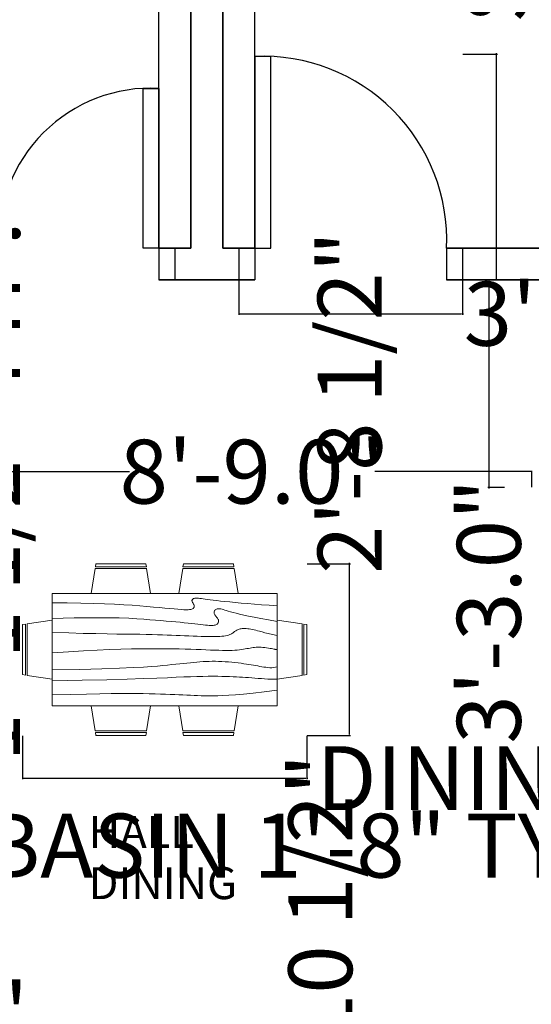
# Model space of a CAD drawing. Units: inches. Extents: x -52 to 472, y -40 to 644.
# Tile 4 of 6: x 154 to 250, y 164 to 349. Entities that reach past the tile are written whole.
import ezdxf

# ---------------------------------------------------------------- set-up
doc = ezdxf.new("R2010")
doc.units = ezdxf.units.IN
doc.header["$MEASUREMENT"] = 0
for name, color, linetype, lineweight in [('A-ANNO-DIMS', 7, 'Continuous', 13), ('A-ANNO-TEXT', 7, 'Continuous', 18), ('DOORS', 2, 'Continuous', 25), ('FURNITURE', 6, 'Continuous', 13), ('INNER WALL', 1, 'Continuous', 35)]:
    doc.layers.add(name, color=color, linetype=linetype, lineweight=lineweight)
doc.styles.get("Standard").update_dxf_attribs({"font": 'arial.ttf'})
doc.dimstyles.get("Standard").update_dxf_attribs({"dimtxt": 12, "dimasz": 0.18, "dimexe": 0.18, "dimexo": 0.0625, "dimgap": 0.09, "dimtad": 0, "dimdec": 1, "dimzin": 0, "dimdsep": 46, "dimlunit": 3, "dimtxsty": 'Standard', "dimcen": 0.09, "dimadec": 0, "dimazin": 0, "dimtfac": 1, "dimtdec": 1, "dimtofl": 0, "dimtmove": 0, "dimatfit": 3, "dimfxl": 1, "dimtolj": 1, "dimtzin": 0, "dimarcsym": 0})

# ---------------------------------------------------------------- blocks, each defined once
blk = doc.blocks.new('Dining Set - 36 x 72 in.')
for p, q in [((-22.2343, 26.00059), (-23.4847, 17.99762)), ((-22.2304, 26), (-5.7608, 26)), ((-22, 27.5), (-22.1562, 26.50042)), ((-5.8416, 26.5), (-22.1534, 26.5)), ((-22, 27.5), (-6, 27.5)), ((-5.8437, 26.49966), (-6, 27.5)), ((-4.5152, 17.99762), (-5.7655, 25.99926)), ((5.7657, 26.00059), (4.5153, 17.99762)), ((5.7696, 26), (22.2392, 26)), ((6, 27.5), (5.8438, 26.50042)), ((22.1584, 26.5), (5.8466, 26.5)), ((6, 27.5), (22, 27.5)), ((22.1563, 26.49966), (22, 27.5)), ((23.4848, 17.99762), (22.2345, 25.99926)), ((36, 18), (-36, 18)), ((-36, 18), (-36, -18)), ((36, -18), (36, 18)), ((-44.0006, 8.23428), (-35.9976, 9.48474)), ((44.0006, 8.23428), (35.9976, 9.48474)), ((-45.5, 8), (-44.5004, 8.15617)), ((-45.5, 8), (-45.5, -8)), ((-44.5, -8.15843), (-44.5, 8.15338)), ((-44, 8.23041), (-44, -8.23915)), ((44, 8.23041), (44, -8.23915)), ((44.5, -8.15843), (44.5, 8.15338)), ((45.5, 8), (44.5005, 8.15617)), ((45.5, 8), (45.5, -8)), ((-44.4997, -8.15631), (-45.5, -8)), ((-35.9976, -9.48476), (-43.9993, -8.2345)), ((35.9976, -9.48476), (43.9993, -8.2345)), ((44.4997, -8.15631), (45.5, -8)), ((-36, -18), (36, -18)), ((-22.2343, -26.0006), (-23.4847, -17.99762)), ((-4.5152, -17.99762), (-5.7655, -25.99928)), ((5.7657, -26.0006), (4.5153, -17.99762)), ((23.4848, -17.99762), (22.2345, -25.99928)), ((-22.2304, -26), (-5.7608, -26)), ((-22, -27.5), (-22.1562, -26.50044)), ((-5.8416, -26.5), (-22.1534, -26.5)), ((-22, -27.5), (-6, -27.5)), ((-5.8437, -26.49967), (-6, -27.5)), ((5.7696, -26), (22.2392, -26)), ((6, -27.5), (5.8438, -26.50044)), ((22.1584, -26.5), (5.8466, -26.5)), ((6, -27.5), (22, -27.5)), ((22.1563, -26.49967), (22, -27.5))]:
    blk.add_line(p, q)
for points in [[(-36, 15), (-31.1772, 14.97754), (-26.8079, 14.91406), (-22.8538, 14.81543), (-19.276, 14.6875), (-16.0362, 14.53613), (-13.0957, 14.36718), (-10.4159, 14.18652), (-7.9583, 14), (-5.6904, 13.81315), (-3.6035, 13.63021), (-1.6954, 13.45508), (0.0365, 13.29166), (1.5945, 13.14388), (2.9811, 13.01562), (4.1988, 12.9108), (5.25, 12.83333), (6.1393, 12.78613), (6.8802, 12.76823), (7.4883, 12.77767), (7.9792, 12.8125), (8.3685, 12.87077), (8.6719, 12.95052), (8.9049, 13.0498), (9.0833, 13.16666), (9.2205, 13.29899), (9.3216, 13.44401), (9.3895, 13.59879), (9.4271, 13.76041), (9.4373, 13.92594), (9.4232, 14.09245), (9.3875, 14.257), (9.3333, 14.41666), (9.2638, 14.56917), (9.1836, 14.71484), (9.0975, 14.85465), (9.0104, 14.98958), (8.9272, 15.1206), (8.8529, 15.2487), (8.7922, 15.37483), (8.75, 15.5), (8.7305, 15.62467), (8.7344, 15.74739), (8.7617, 15.86621), (8.8125, 15.97916), (8.8867, 16.08431), (8.9844, 16.17968), (9.1055, 16.26334), (9.25, 16.33333), (9.4189, 16.38802), (9.6172, 16.42708), (9.8506, 16.45052), (10.125, 16.45833), (10.4463, 16.45052), (10.8203, 16.42708), (11.2529, 16.38802), (11.75, 16.33333), (12.3184, 16.26318), (12.9694, 16.17838), (13.7151, 16.07991), (14.5677, 15.96875), (15.5395, 15.84586), (16.6426, 15.71224), (17.8893, 15.56884), (19.2917, 15.41666), (20.859, 15.25667), (22.5879, 15.08984), (24.4721, 14.91715), (26.5052, 14.73958), (28.6809, 14.5581), (30.9929, 14.3737), (33.4347, 14.18733), (36, 14)], [(-36, 10), (-28.9766, 10.14274), (-23.1725, 10.20442), (-18.4241, 10.19775), (-14.5677, 10.13541), (-11.4399, 10.03011), (-8.877, 9.89453), (-6.7154, 9.74137), (-4.7917, 9.58333), (-2.9698, 9.43082), (-1.2246, 9.28515), (0.4415, 9.14534), (2.026, 9.01041), (3.5266, 8.87939), (4.9408, 8.7513), (6.266, 8.62516), (7.5, 8.5), (8.6411, 8.37549), (9.6914, 8.2539), (10.6538, 8.13818), (11.5312, 8.03125), (12.3267, 7.93603), (13.043, 7.85547), (13.6831, 7.79248), (14.25, 7.75), (14.7471, 7.7303), (15.1797, 7.73307), (15.5537, 7.75732), (15.875, 7.80208), (16.1494, 7.86637), (16.3828, 7.94922), (16.5811, 8.04964), (16.75, 8.16666), (16.8944, 8.29915), (17.0143, 8.44531), (17.1089, 8.60319), (17.1771, 8.77083), (17.218, 8.94629), (17.2305, 9.1276), (17.2137, 9.31282), (17.1667, 9.5), (17.0895, 9.6875), (16.987, 9.875), (16.8649, 10.0625), (16.7292, 10.25), (16.5856, 10.4375), (16.4401, 10.625), (16.2985, 10.8125), (16.1667, 11), (16.05, 11.18733), (15.9518, 11.3737), (15.8752, 11.5581), (15.8229, 11.73958), (15.798, 11.91715), (15.8034, 12.08984), (15.842, 12.25667), (15.9167, 12.41666), (16.0295, 12.56836), (16.1784, 12.70833), (16.3605, 12.83268), (16.5729, 12.9375), (16.8127, 13.01888), (17.0768, 13.07291), (17.3625, 13.0957), (17.6667, 13.08333), (17.9894, 13.03312), (18.3418, 12.94726), (18.7382, 12.82918), (19.1927, 12.68229), (19.7195, 12.51001), (20.3327, 12.31575), (21.0465, 12.10294), (21.875, 11.875), (22.8357, 11.63354), (23.959, 11.37304), (25.2786, 11.08618), (26.8282, 10.76562), (28.6414, 10.40405), (30.752, 9.99414), (33.1936, 9.52856), (36, 9)], [(-36, 5.5), (-30.7157, 5.3348), (-26.069, 5.20963), (-21.9946, 5.11767), (-18.4271, 5.05208), (-15.3009, 5.00602), (-12.5508, 4.97265), (-10.1112, 4.94515), (-7.9167, 4.91666), (-5.909, 4.88167), (-4.0586, 4.83984), (-2.3429, 4.79215), (-0.7396, 4.73958), (0.7739, 4.6831), (2.22, 4.6237), (3.6213, 4.56233), (5, 4.5), (6.373, 4.43782), (7.7344, 4.3776), (9.0723, 4.32129), (10.375, 4.27083), (11.6309, 4.22819), (12.8281, 4.19531), (13.9551, 4.17415), (15, 4.16666), (15.954, 4.17448), (16.819, 4.19791), (17.6001, 4.23698), (18.3021, 4.29166), (18.9299, 4.36198), (19.4883, 4.44791), (19.9823, 4.54948), (20.4167, 4.66666), (20.7969, 4.79899), (21.1302, 4.94401), (21.4245, 5.09879), (21.6875, 5.26041), (21.9271, 5.42594), (22.1511, 5.59245), (22.3672, 5.757), (22.5834, 5.91666), (22.8065, 6.06868), (23.0404, 6.21093), (23.2879, 6.34147), (23.5521, 6.45833), (23.8358, 6.55957), (24.142, 6.64323), (24.4735, 6.70735), (24.8334, 6.75), (25.2235, 6.76969), (25.642, 6.76692), (26.0858, 6.74267), (26.5521, 6.69791), (27.0379, 6.63362), (27.5404, 6.55078), (28.0565, 6.45036), (28.5834, 6.33333), (29.1242, 6.19987), (29.7071, 6.04687), (30.3661, 5.87044), (31.1354, 5.66666), (32.0493, 5.43164), (33.142, 5.16146), (34.4475, 4.85221), (36, 4.5)], [(-36, -1), (-30.7915, -0.6591), (-26.0195, -0.38216), (-21.6519, -0.16284), (-17.6563, 0.00521), (-14.0005, 0.12833), (-10.6523, 0.21289), (-7.5796, 0.26522), (-4.75, 0.29166), (-2.134, 0.29793), (0.2878, 0.28711), (2.5317, 0.26163), (4.6146, 0.22396), (6.5529, 0.17651), (8.3633, 0.12174), (10.0623, 0.06209), (11.6667, 0), (13.1899, -0.06201), (14.6341, -0.1211), (15.9982, -0.17432), (17.2813, -0.21875), (18.4823, -0.25147), (19.6003, -0.26953), (20.6343, -0.27002), (21.5834, -0.25), (22.4481, -0.20768), (23.2357, -0.14584), (23.9549, -0.06836), (24.6146, 0.02083), (25.2235, 0.11784), (25.7904, 0.21875), (26.3241, 0.31966), (26.8334, 0.41666), (27.3265, 0.50618), (27.8099, 0.58593), (28.2894, 0.65397), (28.7709, 0.70833), (29.2601, 0.74707), (29.763, 0.76823), (30.2855, 0.76985), (30.8334, 0.75), (31.4088, 0.70784), (31.9994, 0.64713), (32.589, 0.57275), (33.1615, 0.48958), (33.7008, 0.4025), (34.1908, 0.3164), (34.6153, 0.23616), (34.9584, 0.16666), (35.2099, 0.11165), (35.3848, 0.07031), (35.504, 0.04069), (35.5886, 0.02083), (35.6594, 0.00879), (35.7377, 0.0026), (35.8442, 0.00032), (36, 0)], [(-36, -6.5), (-27.1843, -6.31267), (-20.084, -6.1263), (-14.469, -5.9419), (-10.1094, -5.76042), (-6.7752, -5.58285), (-4.2363, -5.41016), (-2.2629, -5.24333), (-0.625, -5.08334), (0.8708, -4.93099), (2.2715, -4.78646), (3.5872, -4.64974), (4.8281, -4.52084), (6.0046, -4.39974), (7.127, -4.28646), (8.2053, -4.18099), (9.25, -4.08334), (10.2705, -3.99382), (11.2734, -3.91407), (12.2647, -3.84603), (13.25, -3.79167), (14.2354, -3.75293), (15.2266, -3.73177), (16.2295, -3.73015), (17.25, -3.75), (18.2912, -3.79248), (19.3451, -3.85547), (20.4009, -3.93604), (21.4479, -4.03125), (22.4754, -4.13819), (23.4727, -4.25391), (24.4289, -4.37549), (25.3334, -4.5), (26.1785, -4.62492), (26.9694, -4.74935), (27.7145, -4.87281), (28.4219, -4.99479), (29.1, -5.11483), (29.7572, -5.23242), (30.4016, -5.34709), (31.0417, -5.45834), (31.6837, -5.56437), (32.3262, -5.65821), (32.9658, -5.73153), (33.599, -5.77604), (34.2224, -5.78345), (34.8327, -5.74545), (35.4264, -5.65373), (36, -5.5)], [(-36, -10), (-26.4022, -9.81299), (-18.4675, -9.62891), (-11.9839, -9.45069), (-6.7396, -9.28125), (-2.5226, -9.12354), (0.8789, -8.98047), (3.6769, -8.85498), (6.0833, -8.75), (8.2767, -8.66765), (10.3021, -8.60677), (12.1712, -8.56543), (13.8958, -8.54167), (15.4876, -8.53353), (16.9583, -8.53907), (18.3197, -8.55632), (19.5834, -8.58334), (20.7616, -8.61841), (21.8685, -8.66081), (22.9188, -8.71004), (23.9271, -8.76563), (24.9081, -8.82707), (25.8763, -8.89388), (26.8465, -8.96558), (27.8334, -9.04167), (28.8474, -9.12118), (29.8828, -9.20117), (30.93, -9.27824), (31.9792, -9.34896), (33.0205, -9.40991), (34.0443, -9.45768), (35.0407, -9.48885), (36, -9.5)], [(-36, -14.5), (-30.0881, -14.33513), (-25.0332, -14.21224), (-20.7312, -14.12647), (-17.0781, -14.07292), (-13.97, -14.04671), (-11.3027, -14.04297), (-8.9724, -14.05681), (-6.875, -14.08334), (-4.9224, -14.11833), (-3.0905, -14.16016), (-1.3709, -14.20785), (0.2448, -14.26042), (1.7647, -14.3169), (3.1973, -14.3763), (4.5507, -14.43767), (5.8333, -14.5), (7.0554, -14.5621), (8.235, -14.62175), (9.3922, -14.67652), (10.5469, -14.72396), (11.7192, -14.76164), (12.929, -14.78711), (14.1965, -14.79794), (15.5417, -14.79167), (16.9933, -14.76424), (18.6152, -14.70508), (20.4804, -14.60197), (22.6615, -14.44271), (25.2312, -14.21509), (28.2624, -13.9069), (31.8277, -13.50594), (36, -13)]]:
    blk.add_lwpolyline(points)
blk = doc.blocks.new('*D15')
at = {"layer": 'A-ANNO-DIMS', "color": 0, "lineweight": -2, "transparency": 16777216}
for p, q in [((145.13, 258.39), (145.13, 264.49)), ((145.31, 264.31), (174.59, 264.31)), ((249.95, 264.31), (220.67, 264.31)), ((250.13, 261.39), (250.13, 264.49))]:
    blk.add_line(p, q, dxfattribs=at)
at = {"layer": 'A-ANNO-DIMS', "color": 0, "transparency": 16777216}
for points in [[(145.31, 264.34), (145.31, 264.28), (145.13, 264.31)], [(249.95, 264.34), (249.95, 264.28), (250.13, 264.31)]]:
    blk.add_solid(points, dxfattribs=at)
at = {"layer": 'Defpoints', "color": 0, "transparency": 16777216}
for p in [(250.13, 264.31), (250.13, 261.33), (145.13, 258.33)]:
    blk.add_point(p, dxfattribs=at)
at = {"layer": 'A-ANNO-DIMS', "color": 0, "transparency": 16777216, "insert": (197.63, 264.31), "char_height": 12, "attachment_point": 5}
blk.add_mtext('\\A1;8\'-9.0"', dxfattribs=at)
blk = doc.blocks.new('*D17')
at = {"layer": 'A-ANNO-DIMS', "color": 0, "lineweight": -2, "transparency": 16777216}
for p, q in [((32.13, 162.39), (32.13, 162.51)), ((32.31, 162.33), (89.84, 162.33)), ((210.95, 162.33), (153.42, 162.33)), ((211.13, 162.39), (211.13, 162.51))]:
    blk.add_line(p, q, dxfattribs=at)
at = {"layer": 'A-ANNO-DIMS', "color": 0, "transparency": 16777216}
for points in [[(32.31, 162.36), (32.31, 162.3), (32.13, 162.33)], [(210.95, 162.36), (210.95, 162.3), (211.13, 162.33)]]:
    blk.add_solid(points, dxfattribs=at)
at = {"layer": 'Defpoints', "color": 0, "transparency": 16777216}
for p in [(32.13, 162.33), (32.13, 162.33), (211.13, 162.33)]:
    blk.add_point(p, dxfattribs=at)
at = {"layer": 'A-ANNO-DIMS', "color": 0, "transparency": 16777216, "insert": (121.63, 162.33), "char_height": 12, "attachment_point": 5}
blk.add_mtext('\\A1;14\'-11.0"', dxfattribs=at)
blk = doc.blocks.new('*D18')
at = {"layer": 'A-ANNO-DIMS', "color": 0, "lineweight": -2, "transparency": 16777216}
for p, q in [((245, 300.33), (241.89, 300.33)), ((242.07, 300.15), (242.07, 261.49)), ((245, 261.31), (241.89, 261.31)), ((242.07, 261.31), (242.07, 261.13))]:
    blk.add_line(p, q, dxfattribs=at)
at = {"layer": 'A-ANNO-DIMS', "color": 0, "transparency": 16777216}
for points in [[(242.04, 300.15), (242.1, 300.15), (242.07, 300.33)], [(242.04, 261.49), (242.1, 261.49), (242.07, 261.31)]]:
    blk.add_solid(points, dxfattribs=at)
at = {"layer": 'Defpoints', "color": 0, "transparency": 16777216}
for p in [(245.07, 300.33), (242.07, 261.31), (245.07, 261.31)]:
    blk.add_point(p, dxfattribs=at)
at = {"layer": 'A-ANNO-DIMS', "color": 0, "transparency": 16777216, "insert": (242.07, 238.1), "char_height": 12, "attachment_point": 5, "rotation": 90}
blk.add_mtext('\\A1;3\'-3.0"', dxfattribs=at)
blk = doc.blocks.new('DOOR-36IN-SINGLE')
for p, q in [((0, 6), (0, 0)), ((3, 6), (3, 0)), ((39, 6), (39, 0)), ((42, 6), (42, 0))]:
    blk.add_line(p, q)
blk.add_lwpolyline([(3, 6), (6, 6), (6, 42), (3, 42)], close=True)
blk.add_arc((4.5, 7.5), 34.53, 357.5104, 92.4896)
blk = doc.blocks.new('*D32')
at = {"layer": 'A-ANNO-DIMS', "color": 0, "lineweight": -2, "transparency": 16777216}
for p, q in [((125.1, 196.98), (125.1, 193.87)), ((145.03, 196.98), (145.03, 193.87)), ((125.28, 194.05), (144.85, 194.05)), ((145.03, 194.05), (145.21, 194.05))]:
    blk.add_line(p, q, dxfattribs=at)
at = {"layer": 'A-ANNO-DIMS', "color": 0, "transparency": 16777216}
for points in [[(125.28, 194.08), (125.28, 194.02), (125.1, 194.05)], [(144.85, 194.08), (144.85, 194.02), (145.03, 194.05)]]:
    blk.add_solid(points, dxfattribs=at)
at = {"layer": 'Defpoints', "color": 0, "transparency": 16777216}
for p in [(125.1, 197.04), (145.03, 197.04), (145.03, 194.05)]:
    blk.add_point(p, dxfattribs=at)
at = {"layer": 'A-ANNO-DIMS', "color": 0, "transparency": 16777216, "insert": (209.09, 194.05), "char_height": 12, "attachment_point": 5}
blk.add_mtext('\\A1;BASIN 1\'-8" TYP.', dxfattribs=at)
blk = doc.blocks.new('*D33')
at = {"layer": 'A-ANNO-DIMS', "color": 0, "lineweight": -2, "transparency": 16777216}
for p, q in [((145.09, 210.33), (148.2, 210.33)), ((148.02, 210.33), (148.02, 210.51)), ((148.02, 197.22), (148.02, 210.15)), ((145.09, 197.04), (148.2, 197.04))]:
    blk.add_line(p, q, dxfattribs=at)
at = {"layer": 'A-ANNO-DIMS', "color": 0, "transparency": 16777216}
for points in [[(147.99, 210.15), (148.05, 210.15), (148.02, 210.33)], [(147.99, 197.22), (148.05, 197.22), (148.02, 197.04)]]:
    blk.add_solid(points, dxfattribs=at)
at = {"layer": 'Defpoints', "color": 0, "transparency": 16777216}
for p in [(145.03, 210.33), (148.02, 210.33), (145.03, 197.04)]:
    blk.add_point(p, dxfattribs=at)
at = {"layer": 'A-ANNO-DIMS', "color": 0, "transparency": 16777216, "insert": (148.02, 260.59), "char_height": 12, "attachment_point": 5, "rotation": 90}
blk.add_mtext('\\A1;1\'-1 1/2" TYP.', dxfattribs=at)
blk = doc.blocks.new('*D44')
at = {"layer": 'A-ANNO-DIMS', "color": 0, "lineweight": -2, "transparency": 16777216}
for p, q in [((210.42, 92.41), (210.42, 92.59)), ((217.37, 92.41), (210.24, 92.41)), ((210.42, 45.85), (210.42, 92.23)), ((217.37, 45.67), (210.24, 45.67))]:
    blk.add_line(p, q, dxfattribs=at)
at = {"layer": 'A-ANNO-DIMS', "color": 0, "transparency": 16777216}
for points in [[(210.39, 92.23), (210.45, 92.23), (210.42, 92.41)], [(210.39, 45.85), (210.45, 45.85), (210.42, 45.67)]]:
    blk.add_solid(points, dxfattribs=at)
at = {"layer": 'Defpoints', "color": 0, "transparency": 16777216}
for p in [(210.42, 92.41), (217.43, 92.41), (217.43, 45.67)]:
    blk.add_point(p, dxfattribs=at)
at = {"layer": 'A-ANNO-DIMS', "color": 0, "transparency": 16777216, "insert": (210.42, 152.12), "char_height": 12, "attachment_point": 5, "rotation": 90}
blk.add_mtext('\\A1;DESK 3\'-10 1/2"', dxfattribs=at)
blk = doc.blocks.new('*D50')
at = {"layer": 'A-ANNO-DIMS', "color": 0, "lineweight": -2, "transparency": 16777216}
for p, q in [((237.19, 342.75), (243.68, 342.75)), ((243.5, 342.75), (243.5, 342.93)), ((243.5, 300.51), (243.5, 342.57)), ((237.19, 300.33), (243.68, 300.33))]:
    blk.add_line(p, q, dxfattribs=at)
at = {"layer": 'A-ANNO-DIMS', "color": 0, "transparency": 16777216}
for points in [[(243.47, 342.57), (243.53, 342.57), (243.5, 342.75)], [(243.47, 300.51), (243.53, 300.51), (243.5, 300.33)]]:
    blk.add_solid(points, dxfattribs=at)
at = {"layer": 'Defpoints', "color": 0, "transparency": 16777216}
for p in [(237.13, 342.75), (243.5, 342.75), (237.13, 300.33)]:
    blk.add_point(p, dxfattribs=at)
at = {"layer": 'A-ANNO-DIMS', "color": 0, "transparency": 16777216, "insert": (243.5, 454.09), "char_height": 12, "attachment_point": 5, "rotation": 90}
blk.add_mtext('\\A1;SINGLE DOOR 3\'-6 1/2" TYP.', dxfattribs=at)
blk = doc.blocks.new('*D51')
at = {"layer": 'A-ANNO-DIMS', "color": 0, "lineweight": -2, "transparency": 16777216}
for p, q in [((195.13, 300.27), (195.13, 293.79)), ((237.13, 300.27), (237.13, 293.79)), ((195.31, 293.97), (236.95, 293.97)), ((237.13, 293.97), (237.31, 293.97))]:
    blk.add_line(p, q, dxfattribs=at)
at = {"layer": 'A-ANNO-DIMS', "color": 0, "transparency": 16777216}
for points in [[(195.31, 294), (195.31, 293.94), (195.13, 293.97)], [(236.95, 294), (236.95, 293.94), (237.13, 293.97)]]:
    blk.add_solid(points, dxfattribs=at)
at = {"layer": 'Defpoints', "color": 0, "transparency": 16777216}
for p in [(195.13, 300.33), (237.13, 300.33), (237.13, 293.97)]:
    blk.add_point(p, dxfattribs=at)
at = {"layer": 'A-ANNO-DIMS', "color": 0, "transparency": 16777216, "insert": (273.97, 293.97), "char_height": 12, "attachment_point": 5}
blk.add_mtext('\\A1;3\'-6" TYP.', dxfattribs=at)
blk = doc.blocks.new('*D52')
at = {"layer": 'A-ANNO-DIMS', "color": 0, "lineweight": -2, "transparency": 16777216}
for p, q in [((123.77, 136.75), (123.77, 136.93)), ((130.07, 136.75), (123.59, 136.75)), ((123.77, 94.51), (123.77, 136.57)), ((130.07, 94.33), (123.59, 94.33))]:
    blk.add_line(p, q, dxfattribs=at)
at = {"layer": 'A-ANNO-DIMS', "color": 0, "transparency": 16777216}
for points in [[(123.74, 136.57), (123.8, 136.57), (123.77, 136.75)], [(123.74, 94.51), (123.8, 94.51), (123.77, 94.33)]]:
    blk.add_solid(points, dxfattribs=at)
at = {"layer": 'Defpoints', "color": 0, "transparency": 16777216}
for p in [(123.77, 136.75), (130.13, 136.75), (130.13, 94.33)]:
    blk.add_point(p, dxfattribs=at)
at = {"layer": 'A-ANNO-DIMS', "color": 0, "transparency": 16777216, "insert": (123.77, 244.1), "char_height": 12, "attachment_point": 5, "rotation": 90}
blk.add_mtext('\\A1;PAIRED LEAF 3\'-6 1/2" TYP.', dxfattribs=at)
blk = doc.blocks.new('*D53')
at = {"layer": 'A-ANNO-DIMS', "color": 0, "lineweight": -2, "transparency": 16777216}
for p, q in [((130.13, 136.81), (130.13, 143.29)), ((130.31, 143.11), (169.37, 143.11)), ((169.55, 136.81), (169.55, 143.29)), ((169.55, 143.11), (169.73, 143.11))]:
    blk.add_line(p, q, dxfattribs=at)
at = {"layer": 'A-ANNO-DIMS', "color": 0, "transparency": 16777216}
for points in [[(130.31, 143.14), (130.31, 143.08), (130.13, 143.11)], [(169.37, 143.14), (169.37, 143.08), (169.55, 143.11)]]:
    blk.add_solid(points, dxfattribs=at)
at = {"layer": 'Defpoints', "color": 0, "transparency": 16777216}
for p in [(169.55, 143.11), (130.13, 136.75), (169.55, 136.75)]:
    blk.add_point(p, dxfattribs=at)
at = {"layer": 'A-ANNO-DIMS', "color": 0, "transparency": 16777216, "insert": (220.37, 143.11), "char_height": 12, "attachment_point": 5}
blk.add_mtext('\\A1;3\'-3 1/2" TYP.', dxfattribs=at)
blk = doc.blocks.new('*D54')
at = {"layer": 'A-ANNO-DIMS', "color": 0, "lineweight": -2, "transparency": 16777216}
for p, q in [((154.49, 214.67), (154.49, 206.54)), ((207.9, 214.67), (207.9, 206.54)), ((154.67, 206.72), (207.72, 206.72)), ((207.9, 206.72), (208.08, 206.72))]:
    blk.add_line(p, q, dxfattribs=at)
at = {"layer": 'A-ANNO-DIMS', "color": 0, "transparency": 16777216}
for points in [[(154.67, 206.75), (154.67, 206.69), (154.49, 206.72)], [(207.72, 206.75), (207.72, 206.69), (207.9, 206.72)]]:
    blk.add_solid(points, dxfattribs=at)
at = {"layer": 'Defpoints', "color": 0, "transparency": 16777216}
for p in [(154.49, 214.73), (207.9, 214.73), (207.9, 206.72)]:
    blk.add_point(p, dxfattribs=at)
at = {"layer": 'A-ANNO-DIMS', "color": 0, "transparency": 16777216, "insert": (288.1, 206.72), "char_height": 12, "attachment_point": 5}
blk.add_mtext('\\A1;DINING SET 4\'-5 1/2"', dxfattribs=at)
blk = doc.blocks.new('*D55')
at = {"layer": 'A-ANNO-DIMS', "color": 0, "lineweight": -2, "transparency": 16777216}
for p, q in [((207.97, 247.02), (216.1, 247.02)), ((215.92, 247.02), (215.92, 247.2)), ((215.92, 214.91), (215.92, 246.84)), ((207.97, 214.73), (216.1, 214.73))]:
    blk.add_line(p, q, dxfattribs=at)
at = {"layer": 'A-ANNO-DIMS', "color": 0, "transparency": 16777216}
for points in [[(215.89, 246.84), (215.95, 246.84), (215.92, 247.02)], [(215.89, 214.91), (215.95, 214.91), (215.92, 214.73)]]:
    blk.add_solid(points, dxfattribs=at)
at = {"layer": 'Defpoints', "color": 0, "transparency": 16777216}
for p in [(207.9, 247.02), (215.92, 247.02), (207.9, 214.73)]:
    blk.add_point(p, dxfattribs=at)
at = {"layer": 'A-ANNO-DIMS', "color": 0, "transparency": 16777216, "insert": (215.92, 277.32), "char_height": 12, "attachment_point": 5, "rotation": 90}
blk.add_mtext('\\A1;2\'-8 1/2"', dxfattribs=at)
blk = doc.blocks.new('*D80')
at = {"layer": 'A-ANNO-DIMS', "color": 0, "lineweight": -2, "transparency": 16777216}
for p, q in [((150.13, 306.39), (150.13, 508.71)), ((150.31, 508.53), (179.95, 508.53)), ((180.13, 306.39), (180.13, 508.71)), ((180.13, 508.53), (180.31, 508.53))]:
    blk.add_line(p, q, dxfattribs=at)
at = {"layer": 'A-ANNO-DIMS', "color": 0, "transparency": 16777216}
for points in [[(150.31, 508.56), (150.31, 508.5), (150.13, 508.53)], [(179.95, 508.56), (179.95, 508.5), (180.13, 508.53)]]:
    blk.add_solid(points, dxfattribs=at)
at = {"layer": 'Defpoints', "color": 0, "transparency": 16777216}
for p in [(180.13, 508.53), (150.13, 306.33), (180.13, 306.33)]:
    blk.add_point(p, dxfattribs=at)
at = {"layer": 'A-ANNO-DIMS', "color": 0, "transparency": 16777216, "insert": (196.45, 508.53), "char_height": 12, "attachment_point": 5}
blk.add_mtext('\\A1;2\'-6"', dxfattribs=at)
blk = doc.blocks.new('*D81')
at = {"layer": 'A-ANNO-DIMS', "color": 0, "lineweight": -2, "transparency": 16777216}
for p, q in [((180.13, 306.39), (180.13, 508.71)), ((180.31, 508.53), (197.95, 508.53)), ((198.13, 306.39), (198.13, 508.71)), ((198.13, 508.53), (198.31, 508.53))]:
    blk.add_line(p, q, dxfattribs=at)
at = {"layer": 'A-ANNO-DIMS', "color": 0, "transparency": 16777216}
for points in [[(180.31, 508.56), (180.31, 508.5), (180.13, 508.53)], [(197.95, 508.56), (197.95, 508.5), (198.13, 508.53)]]:
    blk.add_solid(points, dxfattribs=at)
at = {"layer": 'Defpoints', "color": 0, "transparency": 16777216}
for p in [(198.13, 508.53), (180.13, 306.33), (198.13, 306.33)]:
    blk.add_point(p, dxfattribs=at)
at = {"layer": 'A-ANNO-DIMS', "color": 0, "transparency": 16777216, "insert": (213.79, 508.53), "char_height": 12, "attachment_point": 5}
blk.add_mtext('\\A1;1\'-6"', dxfattribs=at)

msp = doc.modelspace()

# ---------------------------------------------------------------- linework, layer by layer
at = {"layer": 'DOORS'}
for p, q in [((180.13, 306.33), (180.13, 300.33)), ((183.13, 306.33), (183.13, 300.33))]:
    msp.add_line(p, q, dxfattribs=at)
msp.add_lwpolyline([(180.13, 306.33), (177.13, 306.33), (177.13, 336.33), (180.13, 336.33)], close=True, dxfattribs=at)
msp.add_arc((178.63, 307.83), 28.54, 86.9872, 183.0128, dxfattribs=at)
at = {"layer": 'INNER WALL'}
for p, q in [((186.13, 473.33), (186.13, 306.33)), ((192.13, 473.33), (192.13, 306.33)), ((186.13, 306.33), (180.13, 306.33)), ((198.13, 306.33), (192.13, 306.33)), ((254.13, 306.33), (234.13, 306.33)), ((198.13, 300.33), (180.13, 300.33)), ((344.13, 300.33), (234.13, 300.33))]:
    msp.add_line(p, q, dxfattribs=at)

# ---------------------------------------------------------------- block references
at = {"layer": 'DOORS'}
msp.add_blockref('DOOR-36IN-SINGLE', (195.13, 300.33), dxfattribs=at)
at = {"layer": 'FURNITURE', "xscale": 0.586964509641195, "yscale": 0.586964509641195, "zscale": 0.586964509641195}
msp.add_blockref('Dining Set - 36 x 72 in.', (181.2, 230.87), dxfattribs=at)

# ---------------------------------------------------------------- texts
at = {"layer": 'A-ANNO-TEXT'}
for s, p in [('HALL', (166.89, 193.63)), ('DINING', (166.89, 183.99))]:
    msp.add_text(s, height=6, dxfattribs=at).set_placement(p)

# ---------------------------------------------------------------- dimensions: what is measured, and where the dimension line sits
at = {"layer": 'A-ANNO-DIMS'}
for base, p1, p2, text, picture, middle in [((243.5, 342.75), (237.13, 300.33), (237.13, 342.75), 'SINGLE DOOR <> TYP.', '*D50', (243.5, 454.09)), ((123.77, 136.75), (130.13, 94.33), (130.13, 136.75), 'PAIRED LEAF <> TYP.', '*D52', (123.77, 244.1)), ((148.02, 210.33), (145.03, 197.04), (145.03, 210.33), '<> TYP.', '*D33', (148.02, 260.59)), ((210.42, 92.41), (217.43, 45.67), (217.43, 92.41), 'DESK <>', '*D44', (210.42, 152.12))]:
    dim = msp.add_linear_dim(base=base, p1=p1, p2=p2, angle=90, text=text, dimstyle='Standard', override={"dimdec": 1, "dimlfac": 1, "dimrnd": 0, "dimzin": 1, "dimdsep": 46, "dimlunit": 4, "dimfrac": 2}, dxfattribs=at)
    dim.commit()
    dim.dimension.update_dxf_attribs({"geometry": picture, "text_midpoint": middle})
for base, p1, p2, override, picture, middle in [((180.13, 508.53), (150.13, 306.33), (180.13, 306.33), {"dimdec": 1, "dimlfac": 1, "dimrnd": 0, "dimzin": 1, "dimdsep": 46, "dimlunit": 4, "dimfrac": 2}, '*D80', (196.45, 508.53)), ((198.13, 508.53), (180.13, 306.33), (198.13, 306.33), {"dimdec": 1, "dimlfac": 1, "dimrnd": 0, "dimzin": 1, "dimdsep": 46, "dimlunit": 4, "dimfrac": 2}, '*D81', (213.79, 508.53)), ((250.13, 264.31), (145.13, 258.33), (250.13, 261.33), {"dimclrd": 0, "dimclre": 0, "dimclrt": 0}, '*D15', (197.63, 264.31)), ((32.13, 162.33), (211.13, 162.33), (32.13, 162.33), {"dimclrd": 0, "dimclre": 0, "dimclrt": 0}, '*D17', (121.63, 162.33))]:
    dim = msp.add_linear_dim(base=base, p1=p1, p2=p2, dimstyle='Standard', override=override, dxfattribs=at)
    dim.commit()
    dim.dimension.update_dxf_attribs({"geometry": picture, "text_midpoint": middle})
for base, p1, p2, text, picture, middle in [((237.13, 293.97), (195.13, 300.33), (237.13, 300.33), '<> TYP.', '*D51', (273.97, 293.97)), ((207.9, 206.72), (154.49, 214.73), (207.9, 214.73), 'DINING SET <>', '*D54', (288.1, 206.72)), ((145.03, 194.05), (125.1, 197.04), (145.03, 197.04), 'BASIN <> TYP.', '*D32', (209.09, 194.05)), ((169.55, 143.11), (130.13, 136.75), (169.55, 136.75), '<> TYP.', '*D53', (220.37, 143.11))]:
    dim = msp.add_linear_dim(base=base, p1=p1, p2=p2, text=text, dimstyle='Standard', override={"dimdec": 1, "dimlfac": 1, "dimrnd": 0, "dimzin": 1, "dimdsep": 46, "dimlunit": 4, "dimfrac": 2}, dxfattribs=at)
    dim.commit()
    dim.dimension.update_dxf_attribs({"geometry": picture, "text_midpoint": middle})
for base, p1, p2, override, picture, middle in [((215.92, 247.02), (207.9, 214.73), (207.9, 247.02), {"dimdec": 1, "dimlfac": 1, "dimrnd": 0, "dimzin": 1, "dimdsep": 46, "dimlunit": 4, "dimfrac": 2}, '*D55', (215.92, 277.32)), ((242.07, 261.31), (245.07, 300.33), (245.07, 261.31), {"dimclrd": 0, "dimclre": 0, "dimclrt": 0}, '*D18', (242.07, 238.1))]:
    dim = msp.add_linear_dim(base=base, p1=p1, p2=p2, angle=90, dimstyle='Standard', override=override, dxfattribs=at)
    dim.commit()
    dim.dimension.update_dxf_attribs({"geometry": picture, "text_midpoint": middle})

doc.saveas('drawing.dxf')
